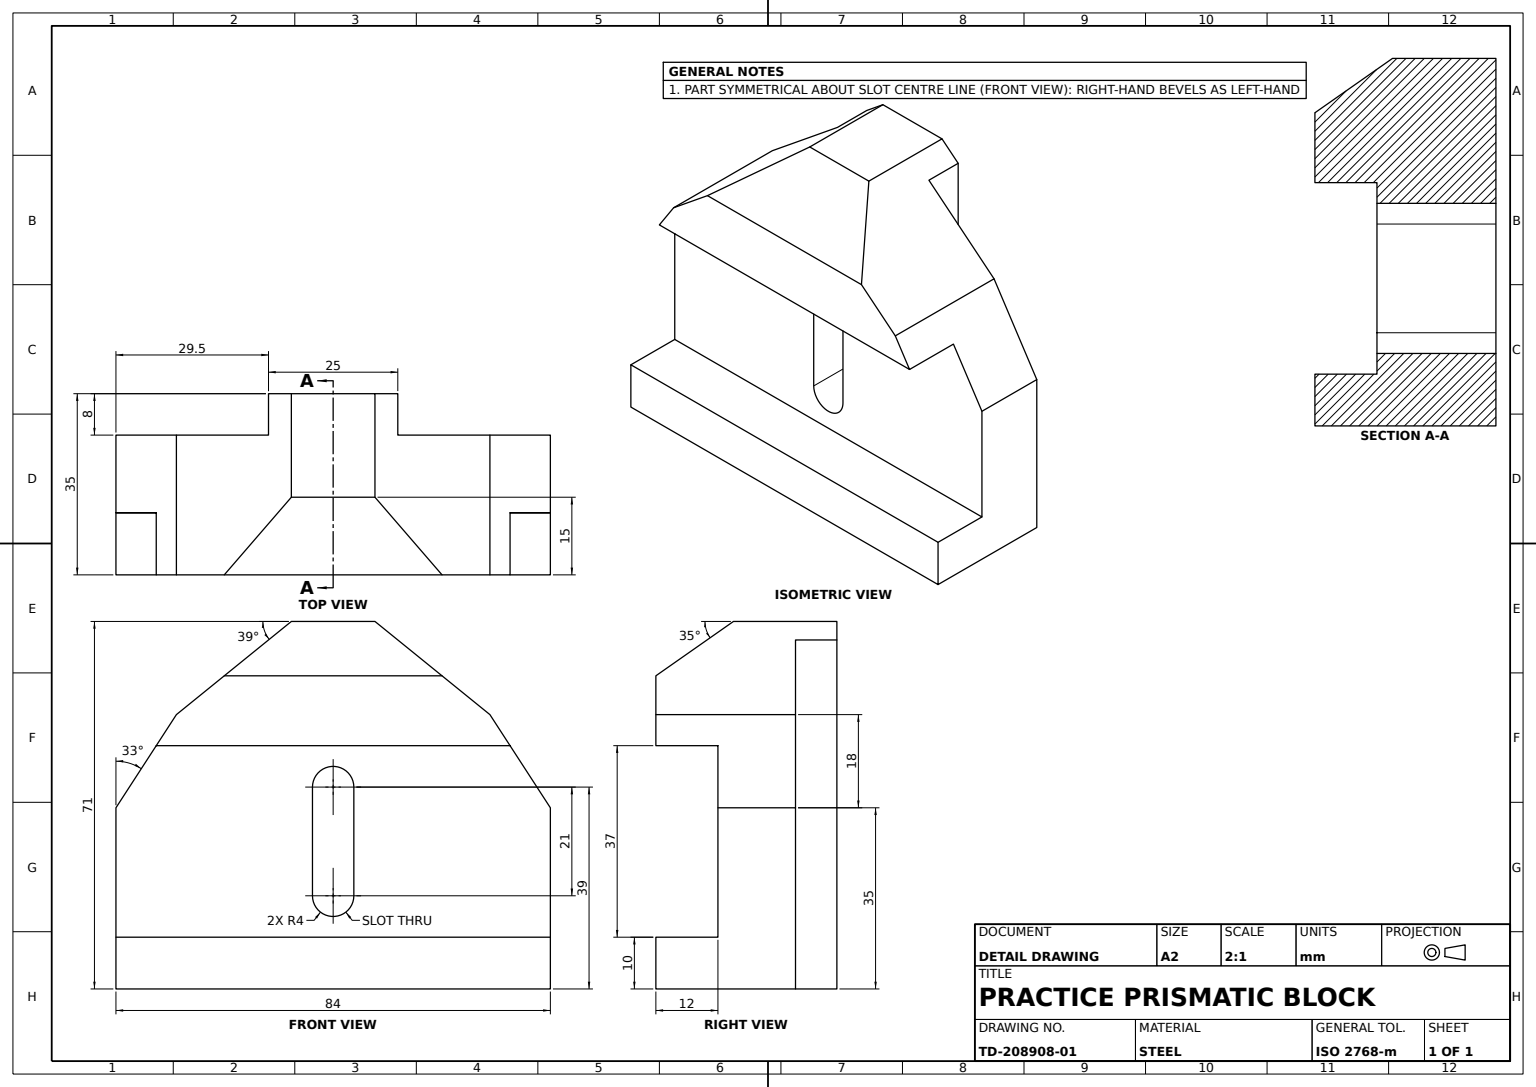
SolidWorks part; units mm, degrees
material "Plain Carbon Steel"
ref_plane "Front Plane" through (0, 0, 0) normal (0, 0, 1) x (1, 0, 0)
ref_plane "Top Plane" through (0, 0, 0) normal (0, 1, 0) x (1, 0, 0)
ref_plane "Right Plane" through (0, 0, 0) normal (1, 0, 0) x (0, 0, -1)
sketch "Block Profile Sketch" plane through (0, 0, 0) normal (1, 0, 0) x (0, 0, -1)
  line L0 (-20, 71) -> (-35, 60.4969)
  line L1 (0, 0) -> (-35, 0)
  line L2 (0, 0) -> (0, 71)
  line L3 (0, 71) -> (-20, 71)
  line L4 (-35, 0) -> (-35, 10)
  line L5 (-35, 60.4969) -> (-35, 47)
  line L6 (-35, 47) -> (-23, 47)
  line L7 (-23, 47) -> (-23, 10)
  line L8 (-23, 10) -> (-35, 10)
  line L9 (-35, 47) -> (-35, 60.4969)
  dimension "D1" = 37
  dimension "D2" = 35
  dimension "D3" = 35
  dimension "D4" = 15
  dimension "D5" = 71
  dimension "D6" = 10
  dimension "D7" = 12
extrude "Support Block 84mm" add sketch "Block Profile Sketch" against normal blind 84 contours L7 L8 L4 L1 L2 L3 L0 L5 L6
sketch "Top Bevel Sketch" plane through (0, 0, 35) normal (0, 0, 1) x (1, 0, 0)
  line L0 (-84, 60.4969) -> (0, 60.4969) construction
  line L1 (0, 47) -> (0, 10) construction
  line L2 (0, 35) -> (-11.6893, 53)
  line L3 (-11.6893, 53) -> (-33.9175, 71)
  line L4 (-84, 71) -> (0, 71) construction
  line L5 (0, 60.4969) -> (0, 47) construction
  line L6 (-50.0825, 71) -> (-95.8763, 71)
  line L8 (-72.3107, 53) -> (-50.0825, 71)
  line L9 (-84, 35) -> (-72.3107, 53)
  line L11 (-95.8763, 71) -> (-95.8763, 33.773)
  line L12 (-95.8763, 33.773) -> (-84, 35)
  line L13 (-33.9175, 71) -> (24.6105, 71)
  line L14 (24.6105, 71) -> (24.6105, 35)
  line L15 (24.6105, 35) -> (0, 35)
  dimension "D1" = 24.6105
  dimension "D2" = 18
  dimension "D3" = 33
  dimension "D4" = 33.9175
  dimension "D5" = 50.0825
  dimension "D6" = 95.8763
  dimension "D7" = 7.4969
  dimension "D8" = 26.7239
extrude "Top Bevel Cut" cut sketch "Top Bevel Sketch" against normal blind 84
sketch "Slot 8mm Sketch" plane through (0, 71, 0) normal (0, 1, 0) x (1, 0, 0)
  line L1 (-84, 0) -> (-54.5, 0)
  line L2 (-84, 0) -> (-84, -8)
  line L3 (-84, -8) -> (-54.5, -8)
  line L4 (-54.5, 0) -> (-54.5, -8)
  line L5 (0, 0) -> (-29.5, 0)
  line L6 (0, 0) -> (0, -8)
  line L7 (0, -8) -> (-29.5, -8)
  line L8 (-29.5, 0) -> (-29.5, -8)
  point P10 (-29.5, -4)
  dimension "D1" = 8
  dimension "D2" = 8
  dimension "D3" = 25
  dimension "D4" = 29.5
extrude "Slot 8mm Cut" cut sketch "Slot 8mm Sketch" against normal blind 104
sketch "Slot 8x21 Sketch" plane through (0, 0, 23) normal (0, 0, 1) x (1, 0, 0)
  line L0 (-42, 0) -> (-42, 74.4448)
  line L1 (-84, 0) -> (0, 0) construction
  line L2 (-42, 18) -> (-42, 39) construction
  line L3 (-46, 18) -> (-46, 39)
  line L4 (-38, 18) -> (-38, 39)
  line L5 (-76.2071, 47) -> (-7.7929, 47) construction
  arc A0 (-46, 18) -> (-38, 18) centre (-42, 18) ccw
  arc A1 (-38, 39) -> (-46, 39) centre (-42, 39) ccw
  point P6 (-42, 28.5)
  dimension "D1" = 21
  dimension "D2" = 8
  dimension "D3" = 39
  dimension "D4" = 27.4448
extrude "Slot 8x21 Cut" cut sketch "Slot 8x21 Sketch" against normal blind 104 contours L4 A1 L3 A0
